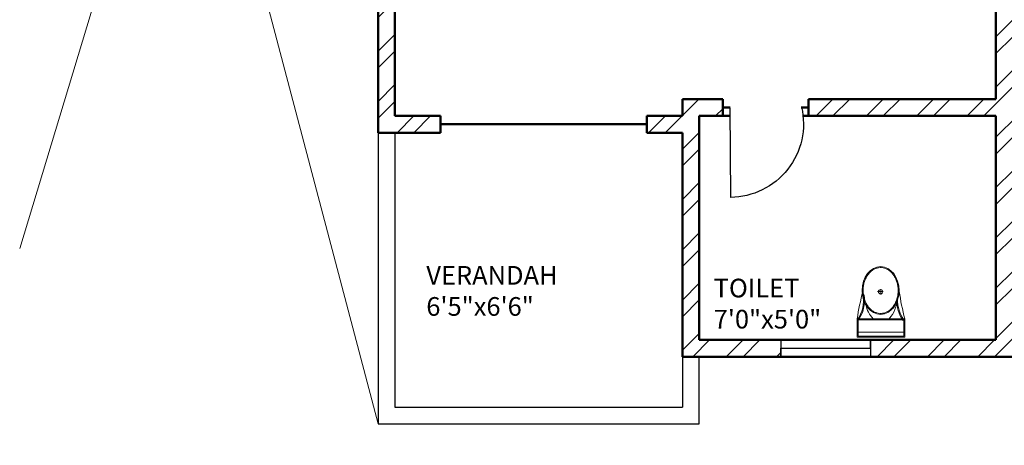
# Model space of a CAD drawing. Units: inches. Extents: x 1901 to 2863, y 888 to 2433.
# Tile 22 of 91: x 2343 to 2607, y 1175 to 1289. Entities that reach past the tile are written whole.
import ezdxf

# ---------------------------------------------------------------- set-up
doc = ezdxf.new("R2010")
doc.units = ezdxf.units.IN
for name, color, linetype, lineweight in [('A-ANNO-SYMB', 8, 'Continuous', 13), ('A-AREA-IDEN', 7, 'Continuous', 18), ('A-DOOR', 4, 'Continuous', 25), ('A-FLOR-FIXT', 9, 'Continuous', 18), ('A-FLOR-HRAL', 41, 'Continuous', 25), ('A-GLAZ', 3, 'Continuous', 25), ('A-WALL', 7, 'Continuous', 50), ('A-WALL-PATT', 8, 'Continuous', 13)]:
    doc.layers.add(name, color=color, linetype=linetype, lineweight=lineweight)
doc.styles.get("Standard").update_dxf_attribs({"font": 'arial.ttf'})

# ---------------------------------------------------------------- blocks, each defined once
blk = doc.blocks.new('A$C31115884')
for p, q in [((283, 498), (223, 498)), ((258, 466), (258, 523)), ((0, 200), (0, 0)), ((520, 200), (0, 200)), ((10, 190), (10, 10)), ((510, 190), (10, 190)), ((510, 10), (510, 190)), ((520, 0), (520, 200)), ((510, 54), (0, 54)), ((10, 10), (510, 10)), ((0, 0), (520, 0))]:
    blk.add_line(p, q)
blk.add_circle((256, 496), 23.6)
for centre, radius, start, end in [((2778, -205), 2807, 165.4549, 171.7133), ((-295, 403), 365, 324.2091, 9.3499), ((-295, 403), 375, 324.2091, 9.3499), ((806, 403), 365, 170.6501, 215.7909), ((3237, 905), 2807, 188.2867, 194.5451), ((384, 406), 293, 190.2774, 224.1564), ((139, 406), 293, 315.8436, 2.6563), ((806, 403), 375, 179.2036, 215.7909)]:
    blk.add_arc(centre, radius, start, end)
blk.add_ellipse((256, 510), major_axis=(0, -261), ratio=0.772727)
blk.add_open_spline([(256, 259), (263, 259), (270, 260), (288, 262), (299, 265), (320, 273), (330, 278), (350, 291), (360, 299), (378, 316), (386, 326), (402, 347), (409, 358), (421, 383), (427, 395), (436, 422), (440, 436), (445, 465), (447, 480), (448, 509), (448, 524), (445, 553), (443, 568), (436, 596), (432, 610), (422, 636), (416, 649), (402, 672), (395, 683), (379, 703), (370, 712), (351, 728), (341, 735), (321, 746), (310, 751), (289, 757), (278, 759), (256, 761), (245, 761), (223, 757), (212, 754), (191, 746), (181, 741), (161, 728), (151, 720), (133, 703), (125, 693), (110, 672), (103, 660), (90, 636), (85, 623), (76, 596), (72, 582), (67, 553), (66, 538), (64, 509), (65, 494), (68, 465), (70, 450), (77, 422), (81, 408), (91, 382), (97, 370), (111, 346), (118, 335), (135, 316), (144, 307), (162, 291), (172, 284), (193, 273), (203, 269), (225, 262), (236, 260), (250, 259), (253, 259), (256, 259)], degree=3, knots=[0, 0, 0, 0, 0.110105, 0.110105, 0.285049, 0.285049, 0.459994, 0.459994, 0.634938, 0.634938, 0.809882, 0.809882, 0.984827, 0.984827, 1.159771, 1.159771, 1.334715, 1.334715, 1.50966, 1.50966, 1.684604, 1.684604, 1.859549, 1.859549, 2.034493, 2.034493, 2.209437, 2.209437, 2.384382, 2.384382, 2.559326, 2.559326, 2.73427, 2.73427, 2.909215, 2.909215, 3.084159, 3.084159, 3.259103, 3.259103, 3.434048, 3.434048, 3.608992, 3.608992, 3.783936, 3.783936, 3.958881, 3.958881, 4.133825, 4.133825, 4.30877, 4.30877, 4.483714, 4.483714, 4.658658, 4.658658, 4.833603, 4.833603, 5.008547, 5.008547, 5.183491, 5.183491, 5.358436, 5.358436, 5.53338, 5.53338, 5.708324, 5.708324, 5.883269, 5.883269, 6.058213, 6.058213, 6.233158, 6.233158, 6.283185, 6.283185, 6.283185, 6.283185])
blk = doc.blocks.new('WIN-24')
for p, q in [((0, 4.5), (0, 0)), ((24, 2.25), (24, 4.5)), ((24, 4.5), (24, 0)), ((0, 0), (0, 2.25)), ((0, 2.25), (24, 2.25))]:
    blk.add_line(p, q)
blk = doc.blocks.new('DOOR-20')
blk.add_line((0, -0.02), (0, 23.98))
blk.add_arc((0, 4.28), 19.71, 347.419, 90)

msp = doc.modelspace()

# ---------------------------------------------------------------- hatches: boundary and pattern name
at = {"layer": 'A-WALL-PATT'}
h = msp.add_hatch(dxfattribs=at)
h.set_pattern_fill('ANSI32', color=256)
h.paths.add_polyline_path([(2192.5, 2274.13), (2141.26, 2274.13), (2141.26, 2269.63), (2192.5, 2269.63)])
h.paths.add_polyline_path([(2259.93, 2274.13), (2216.5, 2274.13), (2216.5, 2269.63), (2255.43, 2269.63), (2255.43, 2214.63), (2250.81, 2214.63), (2250.81, 2210.13), (2259.93, 2210.13), (2259.93, 2215.13), (2271.76, 2215.13), (2271.76, 2217.38), (2271.76, 2219.63), (2259.93, 2219.63)])
h.paths.add_polyline_path([(2171.43, 2269.63), (2166.93, 2269.63), (2166.93, 2219.63), (2121.24, 2219.63), (2121.24, 2215.13), (2166.93, 2215.13), (2166.93, 2083.13), (2161.81, 2083.13), (2161.81, 2078.63), (2171.43, 2078.63), (2177, 2078.63), (2177, 2080.88), (2177, 2083.13), (2171.43, 2083.13), (2171.43, 2210.13), (2230.91, 2210.13), (2230.91, 2212.38), (2230.91, 2214.63), (2171.43, 2214.63)])
h.paths.add_polyline_path([(2117.26, 2274.13), (2089.43, 2274.13), (2089.43, 2219.63), (2081.14, 2219.63), (2081.14, 2215.13), (2089.43, 2215.13), (2098, 2215.13), (2098, 2217.38), (2098, 2219.63), (2093.93, 2219.63), (2093.93, 2269.63), (2117.26, 2269.63), (2117.26, 2271.88)])
h.paths.add_polyline_path([(2343.43, 2219.63), (2329.29, 2219.63), (2329.29, 2215.13), (2338.93, 2215.13), (2338.93, 2184.74), (2343.43, 2184.74)])
h.paths.add_polyline_path([(2338.93, 2083.13), (2329.29, 2083.13), (2208.97, 2083.13), (2208.97, 2078.63), (2338.93, 2078.63)])
h.paths.add_polyline_path([(2343.43, 2136.74), (2338.93, 2136.74), (2338.93, 1872.63), (2343.43, 1872.63)])
h.paths.add_polyline_path([(2343.43, 1863.63), (2397.68, 1863.63), (2397.68, 1821.63), (2384.14, 1821.63), (2384.14, 1812.63), (2418.33, 1812.63), (2418.33, 1817.13), (2418.33, 1821.63), (2406.68, 1821.63), (2406.68, 1863.63), (2459.5, 1863.63), (2459.5, 1821.63), (2447.14, 1821.63), (2447.14, 1812.63), (2459.5, 1812.63), (2468.5, 1812.63), (2468.5, 1872.63), (2394.43, 1872.63), (2334.43, 1872.63), (2334.43, 1812.63), (2343.43, 1812.63), (2353.25, 1812.63), (2353.25, 1821.63), (2343.43, 1821.63)])
h.paths.add_polyline_path([(2510.01, 1872.63), (2468.5, 1872.63), (2468.5, 1868.13), (2510.01, 1868.13)])
h.paths.add_polyline_path([(2514.01, 1817.13), (2468.5, 1817.13), (2468.5, 1812.63), (2482.11, 1812.63), (2482.11, 1800.61), (2486.61, 1800.61), (2486.61, 1812.63), (2514.01, 1812.63)])
h.paths.add_polyline_path([(2299.25, 1814.88), (2299.25, 1817.13), (2295.93, 1817.13), (2295.93, 1854.17), (2293.68, 1854.17), (2291.43, 1854.17), (2291.43, 1817.13), (2266.11, 1817.13), (2266.11, 1812.63), (2299.25, 1812.63)])
h.paths.add_polyline_path([(2218.11, 1817.13), (2206.46, 1817.13), (2171.43, 1817.13), (2171.43, 1949.13), (2190.1, 1949.13), (2190.1, 1953.63), (2163.47, 1953.63), (2163.47, 1949.13), (2166.93, 1949.13), (2166.93, 1817.13), (2114.3, 1817.13), (2114.3, 1812.63), (2218.11, 1812.63)])
h.paths.add_polyline_path([(2029.43, 1970.92), (2024.93, 1970.92), (2024.93, 1912.72), (2029.43, 1912.72)])
h.paths.add_polyline_path([(2132.3, 1953.63), (2113.93, 1953.63), (2113.93, 1975.89), (2111.68, 1975.89), (2109.43, 1975.89), (2109.43, 1953.63), (2029.43, 1953.63), (2029.43, 1949.13), (2132.3, 1949.13)])
h.paths.add_polyline_path([(2029.43, 1853.61), (2029.31, 1853.61), (2029.31, 1853.61), (2029.43, 1853.61), (2029.43, 1864.72), (2024.93, 1864.72), (2024.93, 1812.63), (2066.3, 1812.63), (2066.3, 1814.88), (2066.3, 1817.13), (2029.43, 1817.13)])
h.paths.add_polyline_path([(2122.93, 2010.09), (2120.68, 2010.09), (2118.43, 2010.09), (2118.43, 2006.13), (2029.43, 2006.13), (2029.43, 2001.63), (2109.43, 2001.63), (2109.43, 1998.04), (2113.93, 1998.04), (2113.93, 2001.63), (2122.93, 2001.63)])
h.paths.add_polyline_path([(2029.43, 2031.38), (2024.93, 2031.38), (2024.93, 1994.92), (2027.18, 1994.92), (2029.43, 1994.92)])
h.paths.add_polyline_path([(2029.43, 2136.74), (2024.93, 2136.74), (2024.93, 2067.38), (2027.18, 2067.38), (2029.43, 2067.38)])
h.paths.add_polyline_path([(2125.62, 2083.13), (2029.43, 2083.13), (2029.43, 2078.63), (2118.43, 2078.63), (2118.43, 2030.71), (2122.93, 2030.71), (2122.93, 2078.63), (2125.62, 2078.63)])
h.paths.add_polyline_path([(2029.43, 2215.13), (2040.47, 2215.13), (2040.47, 2217.38), (2040.47, 2219.63), (2024.93, 2219.63), (2024.93, 2184.74), (2029.43, 2184.74), (2029.43, 2187.78)])
h.paths.add_polyline_path([(2686.43, 2274.13), (2659.28, 2274.13), (2659.28, 2269.63), (2681.93, 2269.63), (2681.93, 2219.63), (2676.82, 2219.63), (2676.82, 2215.13), (2681.93, 2215.13), (2697.01, 2215.13), (2697.01, 2217.38), (2697.01, 2219.63), (2686.43, 2219.63)])
h.paths.add_polyline_path([(2609.93, 2269.63), (2635.28, 2269.63), (2635.28, 2274.13), (2571.43, 2274.13), (2571.43, 2269.63), (2605.43, 2269.63), (2605.43, 2214.63), (2549.1, 2214.63), (2549.1, 2210.13), (2605.43, 2210.13), (2605.43, 2083.13), (2601.01, 2083.13), (2601.01, 2080.88), (2601.01, 2078.63), (2609.93, 2078.63), (2616.16, 2078.63), (2616.16, 2080.88), (2616.16, 2083.13), (2609.93, 2083.13), (2609.93, 2215.13), (2651.46, 2215.13), (2651.46, 2217.38), (2651.46, 2219.63), (2609.93, 2219.63)])
h.paths.add_polyline_path([(2521.43, 2269.63), (2547.43, 2269.63), (2547.43, 2271.88), (2547.43, 2274.13), (2516.93, 2274.13), (2516.93, 2219.63), (2506.41, 2219.63), (2506.41, 2215.13), (2516.93, 2215.13), (2516.93, 2210.13), (2525.4, 2210.13), (2525.4, 2212.38), (2525.4, 2214.63), (2521.43, 2214.63)])
h.paths.add_polyline_path([(2456.01, 2219.63), (2439.43, 2219.63), (2439.43, 2187.89), (2443.93, 2187.89), (2443.93, 2215.13), (2456.01, 2215.13)])
h.paths.add_polyline_path([(2752.93, 2219.63), (2739.48, 2219.63), (2739.48, 2215.13), (2748.43, 2215.13), (2748.43, 2187.89), (2752.93, 2187.89)])
h.paths.add_polyline_path([(2752.93, 2139.89), (2748.43, 2139.89), (2748.43, 2083.13), (2648.42, 2083.13), (2648.42, 2078.63), (2654.93, 2078.63), (2654.93, 2039.44), (2659.43, 2039.44), (2659.43, 2078.63), (2748.43, 2078.63), (2748.43, 2063.43), (2752.93, 2063.43)])
h.paths.add_polyline_path([(2752.93, 2010.63), (2659.43, 2010.63), (2659.43, 2015.65), (2654.93, 2015.65), (2654.93, 2010.63), (2605.43, 2010.63), (2605.43, 1920.97), (2609.93, 1920.97), (2609.93, 2006.13), (2748.43, 2006.13), (2748.43, 1982.47), (2752.93, 1982.47)])
h.paths.add_polyline_path([(2752.93, 2027.43), (2748.43, 2027.43), (2748.43, 2010.63), (2752.93, 2010.63)])
h.paths.add_polyline_path([(2748.43, 1886.13), (2609.93, 1886.13), (2609.93, 1889.72), (2605.43, 1889.72), (2605.43, 1861.26), (2609.93, 1861.26), (2609.93, 1881.63), (2748.43, 1881.63)])
h.paths.add_polyline_path([(2456.86, 2228.83), (2498.4, 2228.83), (2498.4, 2247.49), (2456.86, 2247.49)], flags=9)
h.paths.add_polyline_path([(2038.6, 2237.42), (2080.17, 2237.42), (2080.17, 2256.08), (2038.6, 2256.08)], flags=9)
h.paths.add_polyline_path([(2292.01, 1062.39), (2539.93, 1062.39), (2539.93, 1099.49), (2292.01, 1099.49)], flags=9)
h.paths.add_polyline_path([(2424.91, 1832.25), (2448.51, 1832.25), (2448.51, 1846.68), (2424.91, 1846.68)], flags=25)
h.paths.add_polyline_path([(2359.08, 1832.25), (2382.68, 1832.25), (2382.68, 1846.68), (2359.08, 1846.68)], flags=25)
h.paths.add_polyline_path([(2352.9, 1684.8), (2367.54, 1684.8), (2367.54, 1697.17), (2352.9, 1697.17)], flags=9)
h.paths.add_polyline_path([(2079.29, 1755.83), (2169.02, 1755.83), (2169.02, 1774.37), (2079.29, 1774.37)], flags=9)
h.paths.add_polyline_path([(2404.09, 1373.86), (2404.09, 1463.59), (2385.54, 1463.59), (2385.54, 1373.86)], flags=9)
h.paths.add_polyline_path([(2268.09, 2236.37), (2309.64, 2236.37), (2309.64, 2255.03), (2268.09, 2255.03)], flags=9)
h.paths.add_polyline_path([(2575.96, 1700.95), (2665.7, 1700.95), (2665.7, 1719.5), (2575.96, 1719.5)], flags=9)
h.paths.add_polyline_path([(2302.96, 1878.47), (2329.52, 1878.47), (2329.52, 1888.78), (2302.96, 1888.78)], flags=9)
h.paths.add_polyline_path([(2097.42, 2240.58), (2126.57, 2240.58), (2126.57, 2259.23), (2097.42, 2259.23)], flags=9)
h.paths.add_polyline_path([(2208.72, 2246.12), (2237.88, 2246.12), (2237.88, 2264.78), (2208.72, 2264.78)], flags=9)
h.paths.add_polyline_path([(2038.15, 1925.96), (2076.99, 1925.96), (2076.99, 1944.62), (2038.15, 1944.62)], flags=9)
h.paths.add_polyline_path([(2239.14, 1926.67), (2288.46, 1926.67), (2288.46, 1945.33), (2239.14, 1945.33)], flags=9)
h.paths.add_polyline_path([(2175.43, 2007.33), (2212.36, 2007.33), (2212.36, 2025.99), (2175.43, 2025.99)], flags=9)
h.paths.add_polyline_path([(2225.03, 2091.79), (2263.87, 2091.79), (2263.87, 2110.45), (2225.03, 2110.45)], flags=9)
h.paths.add_polyline_path([(2035.4, 2098.48), (2074.24, 2098.48), (2074.24, 2117.14), (2035.4, 2117.14)], flags=9)
h.paths.add_polyline_path([(2050.1, 2029.21), (2083.26, 2029.21), (2083.26, 2047.87), (2050.1, 2047.87)], flags=9)
h.paths.add_polyline_path([(2069.68, 1956.72), (2098.83, 1956.72), (2098.83, 1975.38), (2069.68, 1975.38)], flags=25)
h.paths.add_polyline_path([(2328.62, 1753.34), (2361.66, 1753.34), (2361.66, 1771.99), (2328.62, 1771.99)], flags=9)
h.paths.add_polyline_path([(2395.16, 2060.89), (2395.16, 2140.65), (2378.68, 2140.65), (2378.68, 2060.89)], flags=9)
h.paths.add_polyline_path([(2463.73, 2059.02), (2492.89, 2059.02), (2492.89, 2077.68), (2463.73, 2077.68)], flags=9)
h.paths.add_polyline_path([(2458.03, 2181.54), (2496.87, 2181.54), (2496.87, 2200.19), (2458.03, 2200.19)], flags=9)
h.paths.add_polyline_path([(2527.58, 2243.07), (2556.73, 2243.07), (2556.73, 2261.73), (2527.58, 2261.73)], flags=9)
h.paths.add_polyline_path([(2694.46, 2232.77), (2736.03, 2232.77), (2736.03, 2251.42), (2694.46, 2251.42)], flags=9)
h.paths.add_polyline_path([(2637.82, 2249.22), (2666.98, 2249.22), (2666.98, 2267.88), (2637.82, 2267.88)], flags=9)
h.paths.add_polyline_path([(2623.69, 2183.54), (2662.53, 2183.54), (2662.53, 2202.2), (2623.69, 2202.2)], flags=9)
h.paths.add_polyline_path([(2691.97, 2021.5), (2725.12, 2021.5), (2725.12, 2040.16), (2691.97, 2040.16)], flags=9)
h.paths.add_polyline_path([(2621.04, 1975.91), (2662.34, 1975.91), (2662.34, 1994.57), (2621.04, 1994.57)], flags=25)
h.paths.add_polyline_path([(2479.03, 1927.62), (2519.84, 1927.62), (2519.84, 1946.28), (2479.03, 1946.28)], flags=9)
h.paths.add_polyline_path([(2670.94, 1849.08), (2716.01, 1849.08), (2716.01, 1867.73), (2670.94, 1867.73)], flags=9)
h.paths.add_polyline_path([(2523.61, 1782.96), (2550.17, 1782.96), (2550.17, 1793.26), (2523.61, 1793.26)], flags=9)
h.paths.add_polyline_path([(2450.84, 1207.33), (2492.39, 1207.33), (2492.39, 1225.99), (2450.84, 1225.99)], flags=9)
h.paths.add_polyline_path([(2527.75, 1203.84), (2556.91, 1203.84), (2556.91, 1222.5), (2527.75, 1222.5)], flags=9)
h.paths.add_polyline_path([(2639.11, 1207.2), (2668.27, 1207.2), (2668.27, 1225.86), (2639.11, 1225.86)], flags=9)
h.paths.add_polyline_path([(2692.59, 1218.97), (2734.17, 1218.97), (2734.17, 1237.62), (2692.59, 1237.62)], flags=9)
h.paths.add_polyline_path([(2669.27, 1366.33), (2708.11, 1366.33), (2708.11, 1384.99), (2669.27, 1384.99)], flags=9)
h.paths.add_polyline_path([(2463.31, 1358.03), (2502.15, 1358.03), (2502.15, 1376.69), (2463.31, 1376.69)], flags=9)
h.paths.add_polyline_path([(2494.72, 1449.96), (2531.65, 1449.96), (2531.65, 1468.62), (2494.72, 1468.62)], flags=9)
h.paths.add_polyline_path([(2675.57, 1422.16), (2708.72, 1422.16), (2708.72, 1440.81), (2675.57, 1440.81)], flags=9)
h.paths.add_polyline_path([(2685.63, 1493.89), (2714.79, 1493.89), (2714.79, 1512.55), (2685.63, 1512.55)], flags=9)
h.paths.add_polyline_path([(2686.8, 1529.91), (2725.65, 1529.91), (2725.65, 1548.57), (2686.8, 1548.57)], flags=9)
h.paths.add_polyline_path([(2503.65, 1537.99), (2552.97, 1537.99), (2552.97, 1556.65), (2503.65, 1556.65)], flags=9)
h.paths.add_polyline_path([(2291.71, 1643.5), (2318.28, 1643.5), (2318.28, 1653.81), (2291.71, 1653.81)], flags=9)
h.paths.add_polyline_path([(2450.63, 1610.52), (2477.19, 1610.52), (2477.19, 1620.82), (2450.63, 1620.82)], flags=9)
h.paths.add_polyline_path([(2359.99, 1551.81), (2422.25, 1551.81), (2422.25, 1562.12), (2359.99, 1562.12)], flags=9)
h.paths.add_polyline_path([(2280.11, 1249.01), (2321.65, 1249.01), (2321.65, 1267.66), (2280.11, 1267.66)], flags=9)
h.paths.add_polyline_path([(2164.06, 1274.23), (2193.22, 1274.23), (2193.22, 1292.89), (2164.06, 1292.89)], flags=9)
h.paths.add_polyline_path([(2118.21, 1277.69), (2151.25, 1277.69), (2151.25, 1296.35), (2118.21, 1296.35)], flags=9)
h.paths.add_polyline_path([(2031.95, 1268.53), (2073.52, 1268.53), (2073.52, 1287.19), (2031.95, 1287.19)], flags=9)
h.paths.add_polyline_path([(2050.2, 1409.08), (2089.04, 1409.08), (2089.04, 1427.74), (2050.2, 1427.74)], flags=9)
h.paths.add_polyline_path([(2243.74, 1421.03), (2282.58, 1421.03), (2282.58, 1439.69), (2243.74, 1439.69)], flags=9)
h.paths.add_polyline_path([(2190.75, 1509.77), (2231.56, 1509.77), (2231.56, 1528.43), (2190.75, 1528.43)], flags=9)
h.paths.add_polyline_path([(2058.39, 1475.42), (2091.55, 1475.42), (2091.55, 1494.07), (2058.39, 1494.07)], flags=9)
h.paths.add_polyline_path([(2062.45, 1553.09), (2091.6, 1553.09), (2091.6, 1571.75), (2062.45, 1571.75)], flags=9)
h.paths.add_polyline_path([(2219.52, 1590.37), (2266.15, 1590.37), (2266.15, 1609.02), (2219.52, 1609.02)], flags=9)
h.paths.add_polyline_path([(2041.07, 1584.19), (2079.91, 1584.19), (2079.91, 1602.85), (2041.07, 1602.85)], flags=9)
h = msp.add_hatch(dxfattribs=at)
h.set_pattern_fill('ANSI32', color=256)
h.paths.add_polyline_path([(2443.93, 2139.89), (2439.43, 2139.89), (2439.43, 2069.35), (2441.68, 2069.35), (2443.93, 2069.35), (2443.93, 2078.63), (2521.93, 2078.63), (2521.93, 2075.07), (2524.18, 2075.07), (2526.43, 2075.07), (2526.43, 2078.63), (2571.75, 2078.63), (2571.75, 2080.88), (2571.75, 2083.13), (2443.93, 2083.13)])
h.paths.add_polyline_path([(2526.43, 2054.63), (2524.18, 2054.63), (2521.93, 2054.63), (2521.93, 2030.63), (2443.93, 2030.63), (2443.93, 2045.35), (2439.43, 2045.35), (2439.43, 1983.87), (2443.93, 1983.87), (2443.93, 2026.13), (2521.93, 2026.13), (2526.43, 2026.13)])
h.paths.add_polyline_path([(2443.93, 1923.87), (2439.43, 1923.87), (2439.43, 1872.63), (2443.93, 1872.63)])
h.paths.add_polyline_path([(2636.23, 1766.13), (2609.93, 1766.13), (2609.93, 1779.79), (2605.43, 1779.79), (2605.43, 1766.13), (2486.61, 1766.13), (2486.61, 1770.67), (2482.11, 1770.67), (2482.11, 1766.13), (2482.11, 1761.63), (2636.23, 1761.63), (2636.23, 1763.88)])
h.paths.add_polyline_path([(2519.54, 1663.38), (2519.54, 1665.63), (2494.93, 1665.63), (2481.83, 1665.63), (2481.83, 1663.38), (2481.83, 1661.13), (2490.43, 1661.13), (2490.43, 1640.16), (2494.93, 1640.16), (2494.93, 1661.13), (2519.54, 1661.13)])
h.paths.add_polyline_path([(2443.93, 1712.13), (2443.93, 1716.63), (2414.46, 1716.63), (2414.46, 1712.13), (2439.43, 1712.13), (2439.43, 1545.51), (2443.93, 1545.51), (2443.93, 1661.13), (2448.47, 1661.13), (2448.47, 1665.63), (2443.93, 1665.63)])
h.paths.add_polyline_path([(2343.43, 1712.13), (2365.52, 1712.13), (2365.52, 1714.38), (2365.52, 1716.63), (2333.87, 1716.63), (2333.87, 1714.38), (2333.87, 1712.13), (2338.93, 1712.13), (2338.93, 1575.63), (2338.93, 1545.51), (2343.43, 1545.51), (2343.43, 1547.51), (2343.43, 1580.13)])
h.paths.add_polyline_path([(2752.93, 1665.63), (2579.54, 1665.63), (2579.54, 1661.13), (2615.93, 1661.13), (2615.93, 1529.13), (2598.93, 1529.13), (2598.93, 1524.63), (2623.13, 1524.63), (2623.13, 1526.88), (2623.13, 1529.13), (2620.43, 1529.13), (2620.43, 1661.13), (2748.43, 1661.13), (2748.43, 1633.5), (2752.93, 1633.5)])
h.paths.add_polyline_path([(2752.93, 1419.93), (2748.43, 1419.93), (2748.43, 1400.13), (2659.43, 1400.13), (2659.43, 1444.33), (2657.18, 1444.33), (2654.93, 1444.33), (2654.93, 1400.13), (2643.65, 1400.13), (2643.65, 1395.63), (2748.43, 1395.63), (2748.43, 1364.04), (2752.93, 1364.04)])
h.paths.add_polyline_path([(2752.93, 1492.88), (2748.43, 1492.88), (2748.43, 1476.63), (2667.43, 1476.63), (2667.43, 1479.71), (2665.18, 1479.71), (2662.93, 1479.71), (2662.93, 1476.63), (2654.93, 1476.63), (2654.93, 1469.54), (2659.43, 1469.54), (2659.43, 1472.13), (2748.43, 1472.13), (2748.43, 1455.93), (2752.93, 1455.93)])
h.paths.add_polyline_path([(2752.93, 1304.04), (2748.43, 1304.04), (2748.43, 1263.63), (2738.66, 1263.63), (2738.66, 1259.13), (2752.93, 1259.13)])
h.paths.add_polyline_path([(2685.93, 1259.13), (2695.49, 1259.13), (2695.49, 1261.38), (2695.49, 1263.63), (2677.84, 1263.63), (2677.84, 1261.38), (2677.84, 1259.13), (2681.43, 1259.13), (2681.43, 1203.63), (2653.28, 1203.63), (2653.28, 1199.13), (2685.93, 1199.13), (2685.93, 1203.63)])
h.paths.add_polyline_path([(2609.43, 1395.63), (2611.85, 1395.63), (2611.85, 1400.13), (2598.89, 1400.13), (2598.89, 1397.88), (2598.89, 1395.63), (2604.93, 1395.63), (2604.93, 1268.13), (2554.73, 1268.13), (2554.73, 1265.88), (2554.73, 1263.63), (2604.93, 1263.63), (2604.93, 1203.63), (2571.31, 1203.63), (2571.31, 1199.13), (2604.93, 1199.13), (2629.28, 1199.13), (2629.28, 1201.38), (2629.28, 1203.63), (2609.43, 1203.63), (2609.43, 1258.63), (2609.43, 1259.13), (2654.8, 1259.13), (2654.8, 1263.63), (2609.43, 1263.63)])
h.paths.add_polyline_path([(2443.93, 1304.04), (2439.43, 1304.04), (2439.43, 1259.13), (2443.93, 1259.13), (2456.16, 1259.13), (2456.16, 1261.38), (2456.16, 1263.63), (2443.93, 1263.63)])
h.paths.add_polyline_path([(2525.43, 1263.63), (2531.78, 1263.63), (2531.78, 1268.13), (2520.93, 1268.13), (2520.93, 1263.63), (2511.41, 1263.63), (2511.41, 1259.13), (2520.93, 1259.13), (2520.93, 1199.13), (2547.31, 1199.13), (2547.31, 1201.38), (2547.31, 1203.63), (2525.43, 1203.63)])
h.paths.add_polyline_path([(2443.93, 1434.84), (2439.43, 1434.84), (2439.43, 1364.04), (2441.68, 1364.04), (2443.93, 1364.04)])
h.paths.add_polyline_path([(2567.13, 1400.13), (2443.93, 1400.13), (2443.93, 1395.63), (2567.13, 1395.63)])
h.paths.add_polyline_path([(2443.93, 1545.51), (2439.43, 1545.51), (2439.43, 1494.84), (2443.93, 1494.84)])
h.paths.add_polyline_path([(2494.93, 1553.35), (2492.68, 1553.35), (2490.43, 1553.35), (2490.43, 1524.63), (2494.93, 1524.63), (2525.94, 1524.63), (2525.94, 1526.88), (2525.94, 1529.13), (2494.93, 1529.13)])
h.paths.add_polyline_path([(2752.93, 1573.5), (2748.43, 1573.5), (2748.43, 1529.13), (2657.76, 1529.13), (2657.76, 1524.63), (2662.93, 1524.63), (2662.93, 1498.63), (2667.43, 1498.63), (2667.43, 1524.63), (2748.43, 1524.63), (2748.43, 1516.88), (2752.93, 1516.88)])
h.paths.add_polyline_path([(2038.6, 2237.42), (2080.17, 2237.42), (2080.17, 2256.08), (2038.6, 2256.08)], flags=9)
h.paths.add_polyline_path([(2292.01, 1062.39), (2539.93, 1062.39), (2539.93, 1099.49), (2292.01, 1099.49)], flags=9)
h.paths.add_polyline_path([(2424.91, 1832.25), (2448.51, 1832.25), (2448.51, 1846.68), (2424.91, 1846.68)], flags=9)
h.paths.add_polyline_path([(2359.08, 1832.25), (2382.68, 1832.25), (2382.68, 1846.68), (2359.08, 1846.68)], flags=9)
h.paths.add_polyline_path([(2352.9, 1684.8), (2367.54, 1684.8), (2367.54, 1697.17), (2352.9, 1697.17)], flags=9)
h.paths.add_polyline_path([(2079.29, 1755.83), (2169.02, 1755.83), (2169.02, 1774.37), (2079.29, 1774.37)], flags=9)
h.paths.add_polyline_path([(2404.09, 1373.86), (2404.09, 1463.59), (2385.54, 1463.59), (2385.54, 1373.86)], flags=9)
h.paths.add_polyline_path([(2268.09, 2236.37), (2309.64, 2236.37), (2309.64, 2255.03), (2268.09, 2255.03)], flags=9)
h.paths.add_polyline_path([(2575.96, 1700.95), (2665.7, 1700.95), (2665.7, 1719.5), (2575.96, 1719.5)], flags=9)
h.paths.add_polyline_path([(2302.96, 1878.47), (2329.52, 1878.47), (2329.52, 1888.78), (2302.96, 1888.78)], flags=9)
h.paths.add_polyline_path([(2097.42, 2240.58), (2126.57, 2240.58), (2126.57, 2259.23), (2097.42, 2259.23)], flags=9)
h.paths.add_polyline_path([(2208.72, 2246.12), (2237.88, 2246.12), (2237.88, 2264.78), (2208.72, 2264.78)], flags=9)
h.paths.add_polyline_path([(2038.15, 1925.96), (2076.99, 1925.96), (2076.99, 1944.62), (2038.15, 1944.62)], flags=9)
h.paths.add_polyline_path([(2239.14, 1926.67), (2288.46, 1926.67), (2288.46, 1945.33), (2239.14, 1945.33)], flags=9)
h.paths.add_polyline_path([(2175.43, 2007.33), (2212.36, 2007.33), (2212.36, 2025.99), (2175.43, 2025.99)], flags=9)
h.paths.add_polyline_path([(2225.03, 2091.79), (2263.87, 2091.79), (2263.87, 2110.45), (2225.03, 2110.45)], flags=9)
h.paths.add_polyline_path([(2035.4, 2098.48), (2074.24, 2098.48), (2074.24, 2117.14), (2035.4, 2117.14)], flags=9)
h.paths.add_polyline_path([(2050.1, 2029.21), (2083.26, 2029.21), (2083.26, 2047.87), (2050.1, 2047.87)], flags=9)
h.paths.add_polyline_path([(2069.68, 1956.72), (2098.83, 1956.72), (2098.83, 1975.38), (2069.68, 1975.38)], flags=9)
h.paths.add_polyline_path([(2328.62, 1753.34), (2361.66, 1753.34), (2361.66, 1771.99), (2328.62, 1771.99)], flags=9)
h.paths.add_polyline_path([(2395.16, 2060.89), (2395.16, 2140.65), (2378.68, 2140.65), (2378.68, 2060.89)], flags=9)
h.paths.add_polyline_path([(2463.73, 2059.02), (2492.89, 2059.02), (2492.89, 2077.68), (2463.73, 2077.68)], flags=9)
h.paths.add_polyline_path([(2458.03, 2181.54), (2496.87, 2181.54), (2496.87, 2200.19), (2458.03, 2200.19)], flags=9)
h.paths.add_polyline_path([(2456.86, 2228.83), (2498.4, 2228.83), (2498.4, 2247.49), (2456.86, 2247.49)], flags=9)
h.paths.add_polyline_path([(2527.58, 2243.07), (2556.73, 2243.07), (2556.73, 2261.73), (2527.58, 2261.73)], flags=9)
h.paths.add_polyline_path([(2694.46, 2232.77), (2736.03, 2232.77), (2736.03, 2251.42), (2694.46, 2251.42)], flags=9)
h.paths.add_polyline_path([(2637.82, 2249.22), (2666.98, 2249.22), (2666.98, 2267.88), (2637.82, 2267.88)], flags=9)
h.paths.add_polyline_path([(2623.69, 2183.54), (2662.53, 2183.54), (2662.53, 2202.2), (2623.69, 2202.2)], flags=9)
h.paths.add_polyline_path([(2691.97, 2021.5), (2725.12, 2021.5), (2725.12, 2040.16), (2691.97, 2040.16)], flags=9)
h.paths.add_polyline_path([(2621.04, 1975.91), (2662.34, 1975.91), (2662.34, 1994.57), (2621.04, 1994.57)], flags=9)
h.paths.add_polyline_path([(2479.03, 1927.62), (2519.84, 1927.62), (2519.84, 1946.28), (2479.03, 1946.28)], flags=9)
h.paths.add_polyline_path([(2670.94, 1849.08), (2716.01, 1849.08), (2716.01, 1867.73), (2670.94, 1867.73)], flags=9)
h.paths.add_polyline_path([(2523.61, 1782.96), (2550.17, 1782.96), (2550.17, 1793.26), (2523.61, 1793.26)], flags=9)
h.paths.add_polyline_path([(2450.84, 1207.33), (2492.39, 1207.33), (2492.39, 1225.99), (2450.84, 1225.99)], flags=9)
h.paths.add_polyline_path([(2527.75, 1203.84), (2556.91, 1203.84), (2556.91, 1222.5), (2527.75, 1222.5)], flags=9)
h.paths.add_polyline_path([(2639.11, 1207.2), (2668.27, 1207.2), (2668.27, 1225.86), (2639.11, 1225.86)], flags=9)
h.paths.add_polyline_path([(2692.59, 1218.97), (2734.17, 1218.97), (2734.17, 1237.62), (2692.59, 1237.62)], flags=9)
h.paths.add_polyline_path([(2669.27, 1366.33), (2708.11, 1366.33), (2708.11, 1384.99), (2669.27, 1384.99)], flags=25)
h.paths.add_polyline_path([(2463.31, 1358.03), (2502.15, 1358.03), (2502.15, 1376.69), (2463.31, 1376.69)], flags=9)
h.paths.add_polyline_path([(2494.72, 1449.96), (2531.65, 1449.96), (2531.65, 1468.62), (2494.72, 1468.62)], flags=9)
h.paths.add_polyline_path([(2675.57, 1422.16), (2708.72, 1422.16), (2708.72, 1440.81), (2675.57, 1440.81)], flags=25)
h.paths.add_polyline_path([(2685.63, 1493.89), (2714.79, 1493.89), (2714.79, 1512.55), (2685.63, 1512.55)], flags=9)
h.paths.add_polyline_path([(2686.8, 1529.91), (2725.65, 1529.91), (2725.65, 1548.57), (2686.8, 1548.57)], flags=25)
h.paths.add_polyline_path([(2503.65, 1537.99), (2552.97, 1537.99), (2552.97, 1556.65), (2503.65, 1556.65)], flags=9)
h.paths.add_polyline_path([(2291.71, 1643.5), (2318.28, 1643.5), (2318.28, 1653.81), (2291.71, 1653.81)], flags=9)
h.paths.add_polyline_path([(2450.63, 1610.52), (2477.19, 1610.52), (2477.19, 1620.82), (2450.63, 1620.82)], flags=9)
h.paths.add_polyline_path([(2359.99, 1551.81), (2422.25, 1551.81), (2422.25, 1562.12), (2359.99, 1562.12)], flags=9)
h.paths.add_polyline_path([(2280.11, 1249.01), (2321.65, 1249.01), (2321.65, 1267.66), (2280.11, 1267.66)], flags=9)
h.paths.add_polyline_path([(2164.06, 1274.23), (2193.22, 1274.23), (2193.22, 1292.89), (2164.06, 1292.89)], flags=9)
h.paths.add_polyline_path([(2118.21, 1277.69), (2151.25, 1277.69), (2151.25, 1296.35), (2118.21, 1296.35)], flags=9)
h.paths.add_polyline_path([(2031.95, 1268.53), (2073.52, 1268.53), (2073.52, 1287.19), (2031.95, 1287.19)], flags=9)
h.paths.add_polyline_path([(2050.2, 1409.08), (2089.04, 1409.08), (2089.04, 1427.74), (2050.2, 1427.74)], flags=9)
h.paths.add_polyline_path([(2243.74, 1421.03), (2282.58, 1421.03), (2282.58, 1439.69), (2243.74, 1439.69)], flags=9)
h.paths.add_polyline_path([(2190.75, 1509.77), (2231.56, 1509.77), (2231.56, 1528.43), (2190.75, 1528.43)], flags=9)
h.paths.add_polyline_path([(2058.39, 1475.42), (2091.55, 1475.42), (2091.55, 1494.07), (2058.39, 1494.07)], flags=9)
h.paths.add_polyline_path([(2062.45, 1553.09), (2091.6, 1553.09), (2091.6, 1571.75), (2062.45, 1571.75)], flags=9)
h.paths.add_polyline_path([(2219.52, 1590.37), (2266.15, 1590.37), (2266.15, 1609.02), (2219.52, 1609.02)], flags=9)
h.paths.add_polyline_path([(2041.07, 1584.19), (2079.91, 1584.19), (2079.91, 1602.85), (2041.07, 1602.85)], flags=9)

# ---------------------------------------------------------------- linework, layer by layer
at = {"layer": 'A-ANNO-SYMB'}
for p, q in [((2343.43, 1228.13), (2439.43, 1545.51)), ((2343.43, 1545.51), (2439.43, 1181.13))]:
    msp.add_line(p, q, dxfattribs=at)
at = {"layer": 'A-FLOR-HRAL'}
for p, q in [((2439.43, 1259.13), (2439.43, 1181.13)), ((2443.93, 1259.13), (2443.93, 1185.63)), ((2520.93, 1199.13), (2520.93, 1185.63)), ((2525.43, 1181.13), (2525.43, 1199.13)), ((2443.93, 1185.63), (2520.93, 1185.63)), ((2439.43, 1181.13), (2525.43, 1181.13))]:
    msp.add_line(p, q, dxfattribs=at)
at = {"layer": 'A-WALL'}
for p, q in [((2439.43, 1259.13), (2439.43, 1712.13)), ((2443.93, 1661.13), (2443.93, 1263.63)), ((2604.93, 1395.63), (2604.93, 1268.13)), ((2520.93, 1268.13), (2520.93, 1263.63)), ((2531.78, 1268.13), (2520.93, 1268.13)), ((2531.78, 1263.63), (2531.78, 1268.13)), ((2531.78, 1268.13), (2531.78, 1265.88)), ((2604.93, 1268.13), (2554.73, 1268.13)), ((2554.73, 1263.63), (2554.73, 1268.13)), ((2554.73, 1268.13), (2554.73, 1265.88)), ((2443.93, 1263.63), (2456.16, 1263.63)), ((2456.16, 1263.63), (2456.16, 1259.13)), ((2511.41, 1261.38), (2511.41, 1263.63)), ((2511.41, 1263.63), (2511.41, 1259.13)), ((2511.41, 1263.63), (2520.93, 1263.63)), ((2525.43, 1263.63), (2525.43, 1203.63)), ((2525.43, 1263.63), (2533.78, 1263.63)), ((2531.78, 1265.88), (2533.78, 1265.88)), ((2554.73, 1265.88), (2552.73, 1265.88)), ((2553.12, 1263.63), (2604.93, 1263.63)), ((2604.93, 1203.63), (2604.93, 1263.63)), ((2456.16, 1259.13), (2456.16, 1261.38)), ((2456.16, 1261.38), (2511.41, 1261.38)), ((2443.93, 1259.13), (2439.43, 1259.13)), ((2439.43, 1259.13), (2443.93, 1259.13)), ((2443.93, 1259.13), (2456.16, 1259.13)), ((2511.41, 1259.13), (2520.93, 1259.13)), ((2520.93, 1199.13), (2520.93, 1259.13)), ((2604.93, 1259.13), (2604.93, 1203.63)), ((2525.43, 1203.63), (2604.93, 1203.63)), ((2604.93, 1199.13), (2520.93, 1199.13)), ((2685.93, 1199.13), (2604.93, 1199.13))]:
    msp.add_line(p, q, dxfattribs=at)

# ---------------------------------------------------------------- block references
at = {"layer": 'A-DOOR', "extrusion": (0, 0, -1), "zscale": -1, "rotation": 179.4815950196783}
msp.add_blockref('DOOR-20', (-2533.62, 1265.79), dxfattribs=at)
at = {"layer": 'A-FLOR-FIXT', "xscale": 0.0245149588751191, "yscale": 0.0245149588751191, "zscale": 0.0245149588751191}
msp.add_blockref('A$C31115884', (2567.77, 1204.35), dxfattribs=at)
at = {"layer": 'A-GLAZ'}
msp.add_blockref('WIN-24', (2547.31, 1199.13), dxfattribs=at)

# ---------------------------------------------------------------- texts
at = {"layer": 'A-AREA-IDEN', "char_height": 5, "attachment_point": 1}
for s, width, insert in [('VERANDAH\\P6\'5"x6\'6"', 149.1331, (2452.35, 1223.42)), ('TOILET\\P7\'0"x5\'0"', 82.1858, (2529.33, 1220.01))]:
    msp.add_mtext_dynamic_manual_height_columns(s, width=width, gutter_width=12.5, heights=[0], dxfattribs=dict(at, insert=insert))

doc.saveas('drawing.dxf')
